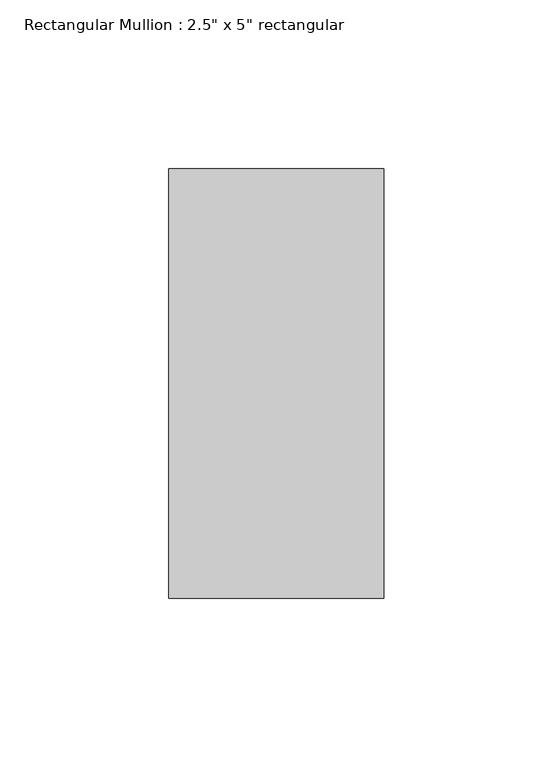
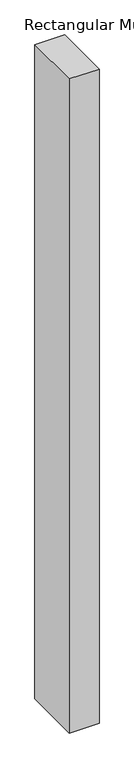
"""IFC4 building model written with IfcOpenShell, lengths in millimetres: member geometry."""

from ifc_helpers import new_model, si_unit, frame, origin, place, context, project, spatial, polyline, outline, extrude, source, transform, mapped, element, save


def member_e79a7e0a(model_context):
    return source(origin(), model_context, "Body", "SweptSolid", [
        extrude(outline(polyline([(0.0, 63.5), (0.0, -63.5), (-63.5, -63.5), (-63.5, 63.5), (0.0, 63.5)])), frame((0.0, 0.0, -1475.8013618), z_axis=(0.0, 0.0, 1.0), x_axis=(1.0, 0.0, 0.0)), (0.0, 0.0, 1.0), 1475.8013618),
    ])


if __name__ == "__main__":
    model = new_model("IFC4")
    model_context = context("Model", 3, world=origin())
    ifc_project = project(units=[si_unit("LENGTHUNIT", "METRE", prefix="MILLI")], contexts=[model_context])
    site = spatial("IfcSite", under=ifc_project)
    building = spatial("IfcBuilding", under=site)
    placement = place(None, origin())
    member_shape = member_e79a7e0a(model_context)
    element("IfcMember", 1, ObjectType="Rectangular Mullion : 2.5\" x 5\" rectangular", at=placement, inside=building, context=model_context, shape_type="MappedRepresentation", body=[
        mapped(member_shape, transform((0.0, 0.0, 0.0), x_axis=(1.0, 0.0, 0.0), y_axis=(0.0, 1.0, 0.0), z_axis=(0.0, 0.0, 1.0))),
    ])
    save(model, "model.ifc")

# Revit data of these elements
# Type "Rectangular Mullion : 2.5\" x 5\" rectangular"
#   built-in parameter 1007304 = 0.416667 (stored number, unit not read)
#   built-in parameter 1007301 = 0.104167 (stored number, unit not read)
#   built-in parameter 1007300 = 0.104167 (stored number, unit not read)
# Element 1 (IfcMember, "Rectangular Mullion : 2.5\" x 5\" rectangular")
#   Materials on its faces: "Aluminum"
# Materials
#   "Aluminum": class "Metal", colour RGB 247 247 247, transparency 0, Description = "Aluminum 6061", Cost = 0
